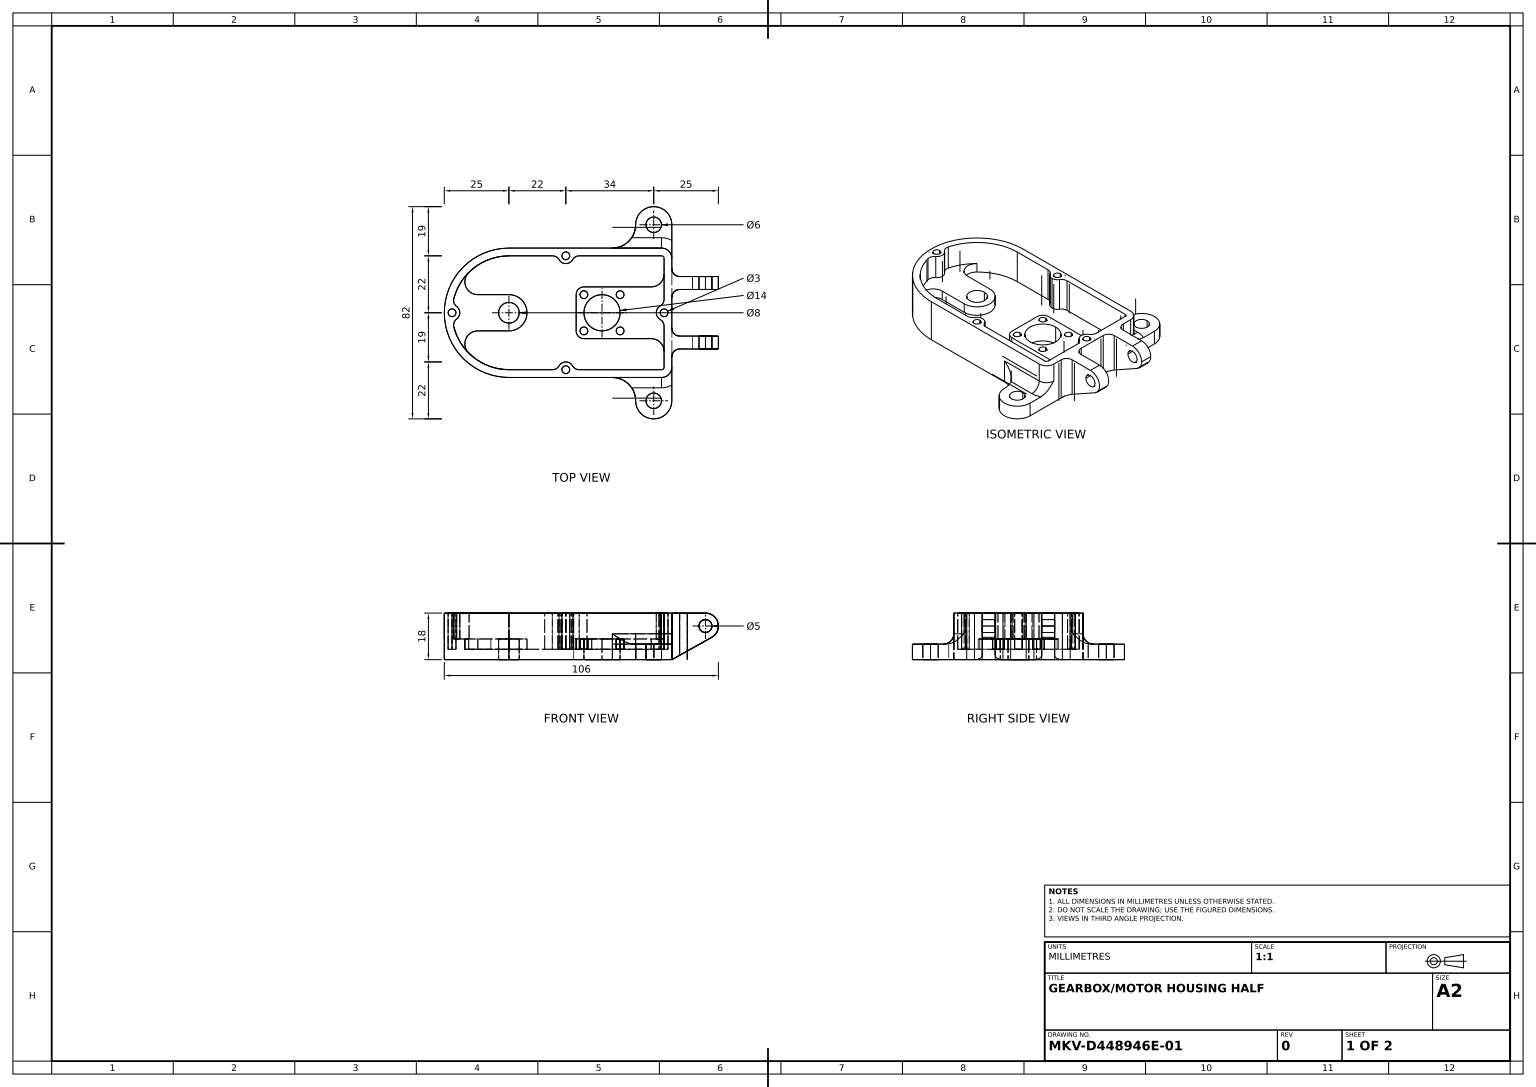
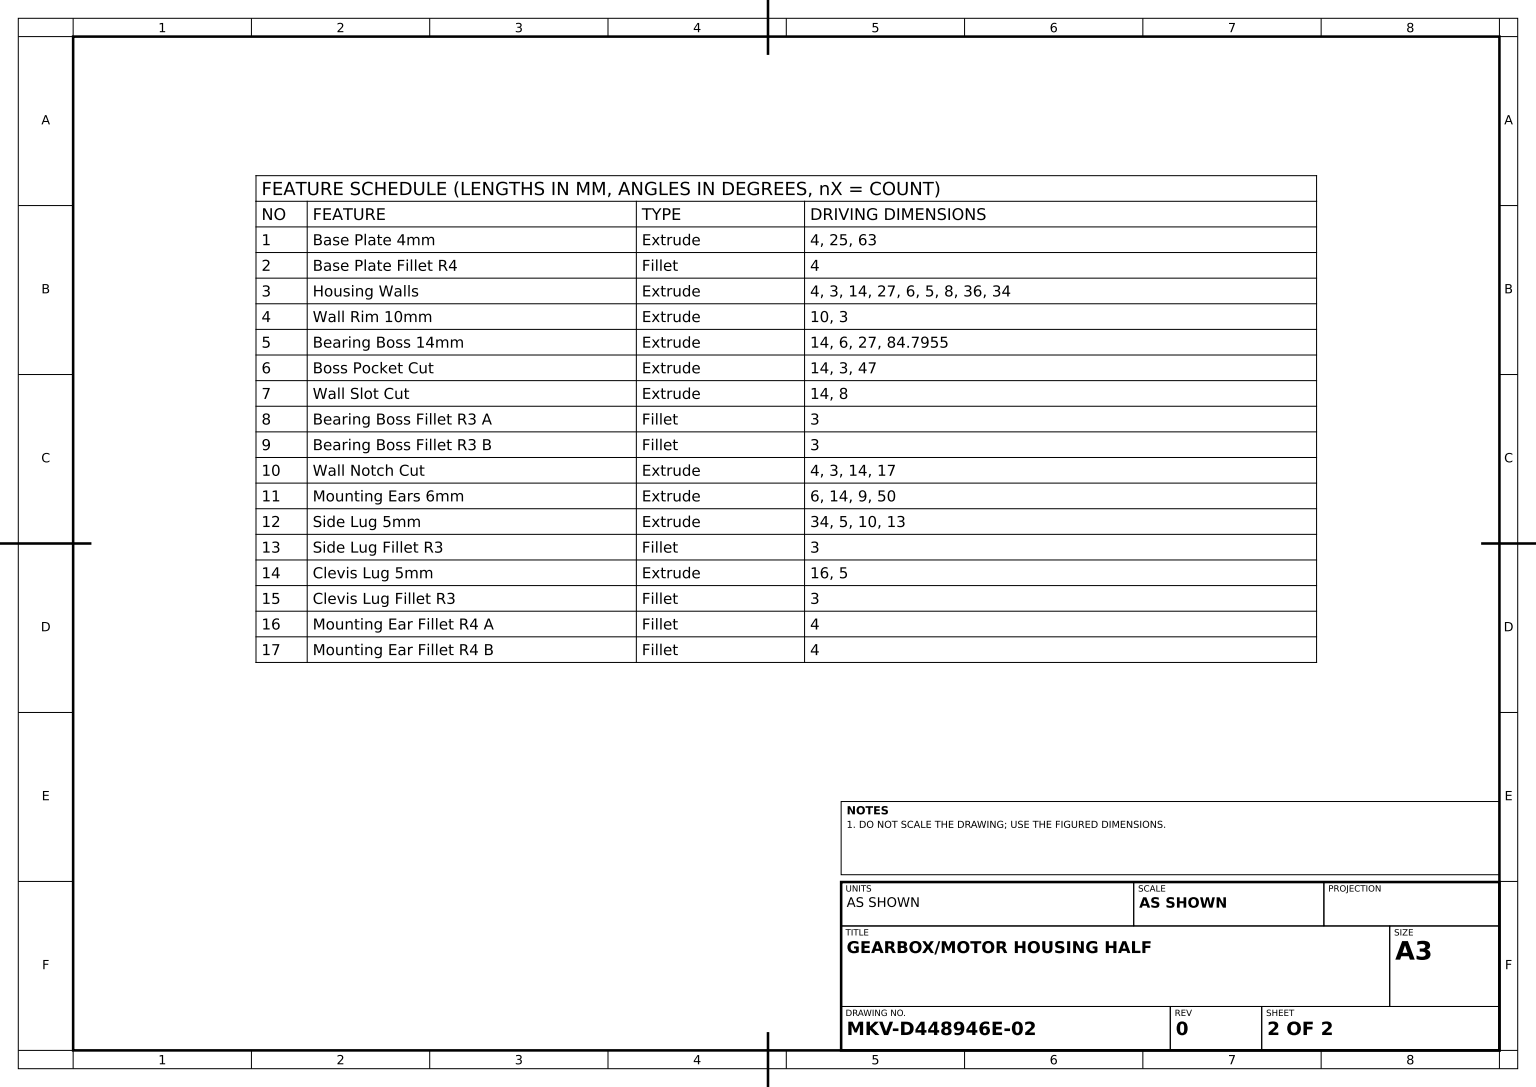
from build123d import *
from build123d.topology import SkipClean

# Parameters (mm, degrees)
BASE_PLATE_4MM_DEPTH       = 4
BASE_PLATE_FILLET_R4_R     = 4
HOUSING_START              = 4
HOUSING_WALL_SKETCH_R      = 7
HOUSING_WALL_SKETCH_R_2    = 4
HOUSING_WALLS_DEPTH        = 4
WALL_START                 = 10
WALL_RIM_10MM_DEPTH        = 10
BEARING_BOSS_14MM_DEPTH    = 14
BOSS_POCKET_SKETCH_R       = 1.5
BOSS_POCKET_CUT_DEPTH      = 14
WALL_SLOT_SKETCH_R         = 4
WALL_SLOT_SKETCH_R_2       = 7
WALL_SLOT_CUT_DEPTH        = 14
BEARING_BOSS_FILLET_R3_A_R = 3
BEARING_BOSS_FILLET_R3_B_R = 3
WALL_NOTCH_SKETCH_R        = 1.5
WALL_NOTCH_CUT_DEPTH       = 4
MOUNTING_START             = -6
MOUNTING_EAR_SKETCH_R      = 3
MOUNTING_EARS_6MM_DEPTH    = 6
SIDE_LUG_SKETCH_R          = 2.5
SIDE_LUG_5MM_DEPTH         = 5
SIDE_LUG_FILLET_R3_R       = 3
CLEVIS_START               = 5
CLEVIS_LUG_SKETCH_R        = 2.5
CLEVIS_LUG_5MM_DEPTH       = 5
CLEVIS_LUG_FILLET_R3_R     = 3
MOUNTING_EAR_FILLET_R4_A_R = 4
MOUNTING_EAR_FILLET_R4_B_R = 4


with BuildPart() as part:
    # Base Plate Sketch → Base Plate 4mm (new body)
    with BuildSketch(Plane(origin=(0, 0, 0), x_dir=(1, 0, 0), z_dir=(0, 1, 0))):
        with BuildLine():
            Line((0, 0), (-63, 0))
            ThreePointArc((-63, 0), (-88, 25), (-63, 50))
            Line((-63, 50), (0, 50))
            Line((0, 50), (0, 0))
        make_face()
    extrude(amount=BASE_PLATE_4MM_DEPTH)

    # Base Plate Fillet R4
    base_plate_fillet_r4_edges = [part.edges().sort_by_distance(p)[0] for p in [
        (0, 2, 0),
        (0, 2, -50),
    ]]
    fillet(base_plate_fillet_r4_edges, radius=BASE_PLATE_FILLET_R4_R)

    # Housing Wall Sketch → Housing Walls (add)
    # profile 1 of 4: a face of its own
    with BuildSketch(Plane(origin=(0, 4, 0), x_dir=(1, 0, 0), z_dir=(0, 1, 0)).offset(HOUSING_START)):
        with BuildLine():
            ThreePointArc((-4, 0), (-1.171572875, 1.171572875), (0, 4))
            Line((0, 4), (0, 46))
            ThreePointArc((0, 46), (-1.171572875, 48.828427125), (-4, 50))
            Line((-4, 50), (-63, 50))
            ThreePointArc((-63, 50), (-88, 25), (-63, 0))
            Line((-63, 0), (-4, 0))
        make_face()
        with BuildLine():
            Line((-63, 47), (-4, 47))
            ThreePointArc((-4, 47), (-3.292893219, 46.707106781), (-3, 46))
            Line((-3, 46), (-3, 4))
            ThreePointArc((-3, 4), (-3.292893219, 3.292893219), (-4, 3))
            Line((-4, 3), (-63, 3))
            ThreePointArc((-63, 3), (-85, 25), (-63, 47))
        make_face(mode=Mode.SUBTRACT)
    # profile 2 of 4: a face of its own
    with BuildSketch(Plane(origin=(0, 4, 0), x_dir=(1, 0, 0), z_dir=(0, 1, 0)).offset(HOUSING_START)):
        with BuildLine():
            ThreePointArc((-8, 15), (-4.464466094, 13.535533906), (-3, 10))
            Line((-3, 10), (-3, 40))
            ThreePointArc((-3, 40), (-4.464466094, 36.464466094), (-8, 35))
            Line((-8, 35), (-34, 35))
            ThreePointArc((-34, 35), (-36.121320344, 34.121320344), (-37, 32))
            Line((-37, 32), (-37, 18))
            ThreePointArc((-37, 18), (-36.121320344, 15.878679656), (-34, 15))
            Line((-34, 15), (-8, 15))
        make_face()
        with Locations(Location((-27, 25, 0), (0, 0, 270))):
            Circle(HOUSING_WALL_SKETCH_R, mode=Mode.SUBTRACT)
    # profile 3 of 4: a face of its own
    with BuildSketch(Plane(origin=(0, 4, 0), x_dir=(1, 0, 0), z_dir=(0, 1, 0)).offset(HOUSING_START)):
        with Locations((-63, 25)):
            Circle(HOUSING_WALL_SKETCH_R)
        with Locations(Location((-63, 25, 0), (0, 0, 270))):
            Circle(HOUSING_WALL_SKETCH_R_2, mode=Mode.SUBTRACT)
    # profile 4 of 4: a face of its own
    with BuildSketch(Plane(origin=(0, 4, 0), x_dir=(1, 0, 0), z_dir=(0, 1, 0)).offset(HOUSING_START)):
        with BuildLine():
            ThreePointArc((-78.583240043, 40.529411765), (-85, 25), (-78.583240043, 9.470588235))
            ThreePointArc((-78.583240043, 9.470588235), (-79.659335305, 14.917412472), (-75.041594579, 18))
            Line((-75.041594579, 18), (-63, 18))
            ThreePointArc((-63, 18), (-70, 25), (-63, 32))
            Line((-63, 32), (-75.041594579, 32))
            ThreePointArc((-75.041594579, 32), (-79.659335305, 35.082587528), (-78.583240043, 40.529411765))
        make_face()
    extrude(amount=-HOUSING_WALLS_DEPTH)

    # Wall Rim Sketch → Wall Rim 10mm (add)
    with SkipClean():  # the faces are left unmerged after this step: merging them gives an invalid solid
        with BuildSketch(Plane(origin=(0, 8, 0), x_dir=(1, 0, 0), z_dir=(0, 1, 0)).offset(WALL_START)):
            with BuildLine():
                Line((-63, 50), (-4, 50))
                ThreePointArc((-4, 50), (-1.171572875, 48.828427125), (0, 46))
                Line((0, 46), (0, 4))
                ThreePointArc((0, 4), (-1.171572875, 1.171572875), (-4, 0))
                Line((-4, 0), (-63, 0))
                ThreePointArc((-63, 0), (-88, 25), (-63, 50))
            make_face()
            with BuildLine():
                Line((-63, 3), (-4, 3))
                ThreePointArc((-4, 3), (-3.292893219, 3.292893219), (-3, 4))
                Line((-3, 4), (-3, 46))
                ThreePointArc((-3, 46), (-3.292893219, 46.707106781), (-4, 47))
                Line((-4, 47), (-63, 47))
                ThreePointArc((-63, 47), (-85, 25), (-63, 3))
            make_face(mode=Mode.SUBTRACT)
        extrude(amount=-WALL_RIM_10MM_DEPTH)

    # Bearing Boss Sketch → Bearing Boss 14mm (add)
    with BuildSketch(Plane(origin=(0, 18, 0), x_dir=(1, 0, 0), z_dir=(0, 1, 0))):
        with BuildLine():
            ThreePointArc((-84.795454545, 22.006981264), (-82, 25), (-84.795454545, 27.993018736))
            ThreePointArc((-84.795454545, 27.993018736), (-85, 25), (-84.795454545, 22.006981264))
        make_face()
        with BuildLine():
            ThreePointArc((-38, 3), (-41, 6), (-44, 3))
            Line((-44, 3), (-38, 3))
        make_face()
        with BuildLine():
            Line((-3, 22), (-3, 28))
            ThreePointArc((-3, 28), (-6, 25), (-3, 22))
        make_face()
        with BuildLine():
            Line((-38, 47), (-44, 47))
            ThreePointArc((-44, 47), (-41, 44), (-38, 47))
        make_face()
    extrude(amount=-BEARING_BOSS_14MM_DEPTH)

    # Boss Pocket Sketch → Boss Pocket Cut (cut)
    with BuildSketch(Plane(origin=(0, 18, 0), x_dir=(1, 0, 0), z_dir=(0, 1, 0))):
        with Locations(Location((-85, 25, 0), (0, 0, 270))):
            Circle(BOSS_POCKET_SKETCH_R)
        with Locations(Location((-41, 3, 0), (0, 0, 90))):
            Circle(BOSS_POCKET_SKETCH_R)
        with Locations(Location((-41, 47, 0), (0, 0, 270))):
            Circle(BOSS_POCKET_SKETCH_R)
        with Locations(Location((-3, 25, 0), (0, 0, 270))):
            Circle(BOSS_POCKET_SKETCH_R)
    extrude(amount=-BOSS_POCKET_CUT_DEPTH, mode=Mode.SUBTRACT)

    # Wall Slot Sketch → Wall Slot Cut (cut)
    with BuildSketch(Plane(origin=(0, 4, 0), x_dir=(1, 0, 0), z_dir=(0, 1, 0))):
        with Locations(Location((-63, 25, 0), (0, 0, 270))):
            Circle(WALL_SLOT_SKETCH_R)
        with Locations(Location((-27, 25, 0), (0, 0, 270))):
            Circle(WALL_SLOT_SKETCH_R_2)
    extrude(amount=-WALL_SLOT_CUT_DEPTH, mode=Mode.SUBTRACT)

    # Bearing Boss Fillet R3 A
    bearing_boss_fillet_r3_a_edges = [part.edges().sort_by_distance(p)[0] for p in [
        (-84.795454545, 13, -22.006981264),
        (-84.795454545, 13, -27.993018736),
    ]]
    fillet(bearing_boss_fillet_r3_a_edges, radius=BEARING_BOSS_FILLET_R3_A_R)

    # Bearing Boss Fillet R3 B
    bearing_boss_fillet_r3_b_edges = [part.edges().sort_by_distance(p)[0] for p in [
        (-38, 11, -3),
        (-44, 11, -3),
        (-3, 13, -28),
        (-3, 13, -22),
        (-44, 11, -47),
        (-38, 11, -47),
    ]]
    fillet(bearing_boss_fillet_r3_b_edges, radius=BEARING_BOSS_FILLET_R3_B_R)

    # Wall Notch Sketch → Wall Notch Cut (cut)
    with BuildSketch(Plane(origin=(0, 8, 0), x_dir=(1, 0, 0), z_dir=(0, 1, 0))):
        with Locations(Location((-34, 32, 0), (0, 0, 270))):
            Circle(WALL_NOTCH_SKETCH_R)
        with Locations(Location((-20, 32, 0), (0, 0, 270))):
            Circle(WALL_NOTCH_SKETCH_R)
        with Locations(Location((-20, 18, 0), (0, 0, 90))):
            Circle(WALL_NOTCH_SKETCH_R)
        with Locations(Location((-34, 18, 0), (0, 0, 90))):
            Circle(WALL_NOTCH_SKETCH_R)
    extrude(amount=-WALL_NOTCH_CUT_DEPTH, mode=Mode.SUBTRACT)

    # Mounting Ear Sketch → Mounting Ears 6mm (add)
    # profile 1 of 2: a face of its own
    with BuildSketch(Plane.XZ.offset(MOUNTING_START)):
        with BuildLine():
            Line((0, 9), (0, -4))
            ThreePointArc((0, -4), (-1.171572875, -1.171572875), (-4, 0))
            Line((-4, 0), (-23, 0))
            ThreePointArc((-23, 0), (-16.636038969, 2.636038969), (-14, 9))
            ThreePointArc((-14, 9), (-7, 16), (0, 9))
        make_face()
        with Locations(Location((-7, 9, 0), (0, 0, 270))):
            Circle(MOUNTING_EAR_SKETCH_R, mode=Mode.SUBTRACT)
    # profile 2 of 2: a face of its own
    with BuildSketch(Plane.XZ.offset(MOUNTING_START)):
        with BuildLine():
            Line((-23, -50), (-4, -50))
            ThreePointArc((-4, -50), (-1.171572875, -48.828427125), (0, -46))
            Line((0, -46), (0, -59))
            ThreePointArc((0, -59), (-7, -66), (-14, -59))
            ThreePointArc((-14, -59), (-16.636038969, -52.636038969), (-23, -50))
        make_face()
        with Locations(Location((-7, -59, 0), (0, 0, 90))):
            Circle(MOUNTING_EAR_SKETCH_R, mode=Mode.SUBTRACT)
    extrude(amount=MOUNTING_EARS_6MM_DEPTH)

    # Side Lug Sketch → Side Lug 5mm (add)
    with BuildSketch(Plane.XY.offset(-34)):
        with BuildLine():
            Line((0, 18), (13, 18))
            ThreePointArc((13, 18), (17.838338777, 14.261141498), (15.440731926, 8.636191151))
            Line((15.440731926, 8.636191151), (0, 0))
            Line((0, 0), (0, 18))
        make_face()
        with Locations((13, 13)):
            Circle(SIDE_LUG_SKETCH_R, mode=Mode.SUBTRACT)
    extrude(amount=-SIDE_LUG_5MM_DEPTH)

    # Side Lug Fillet R3
    side_lug_fillet_r3_edges = [part.edges().sort_by_distance(p)[0] for p in [
        (0, 9, -39),
        (0, 9, -34),
    ]]
    fillet(side_lug_fillet_r3_edges, radius=SIDE_LUG_FILLET_R3_R)

    # Clevis Lug Sketch → Clevis Lug 5mm (add)
    with BuildSketch(Plane.XY.offset(-16).offset(CLEVIS_START)):
        with BuildLine():
            Line((0, 18), (0, 0))
            Line((0, 0), (15.440731926, 8.636191151))
            ThreePointArc((15.440731926, 8.636191151), (17.838338777, 14.261141498), (13, 18))
            Line((13, 18), (0, 18))
        make_face()
        with Locations((13, 13)):
            Circle(CLEVIS_LUG_SKETCH_R, mode=Mode.SUBTRACT)
    extrude(amount=-CLEVIS_LUG_5MM_DEPTH)

    # Clevis Lug Fillet R3
    clevis_lug_fillet_r3_edges = [part.edges().sort_by_distance(p)[0] for p in [
        (0, 9, -11),
        (0, 9, -16),
    ]]
    fillet(clevis_lug_fillet_r3_edges, radius=CLEVIS_LUG_FILLET_R3_R)

    # Mounting Ear Fillet R4 A
    mounting_ear_fillet_r4_a_edges = [part.edges().sort_by_distance(p)[0] for p in [
        (-1.171572875, 6, -1.171572875),
        (-13.5, 6, 0),
    ]]
    fillet(mounting_ear_fillet_r4_a_edges, radius=MOUNTING_EAR_FILLET_R4_A_R)

    # Mounting Ear Fillet R4 B
    mounting_ear_fillet_r4_b_edges = [part.edges().sort_by_distance(p)[0] for p in [
        (-13.5, 6, -50),
        (-1.171572875, 6, -48.828427125),
    ]]
    fillet(mounting_ear_fillet_r4_b_edges, radius=MOUNTING_EAR_FILLET_R4_B_R)


solid = part.part
